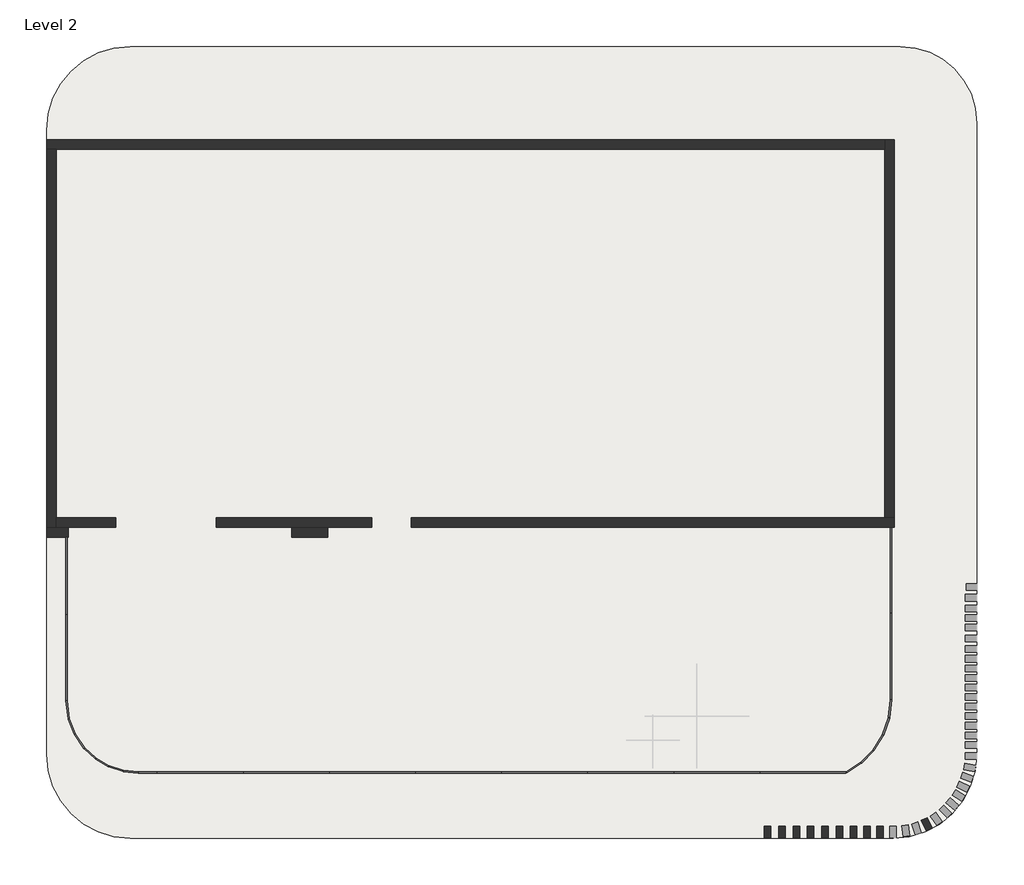
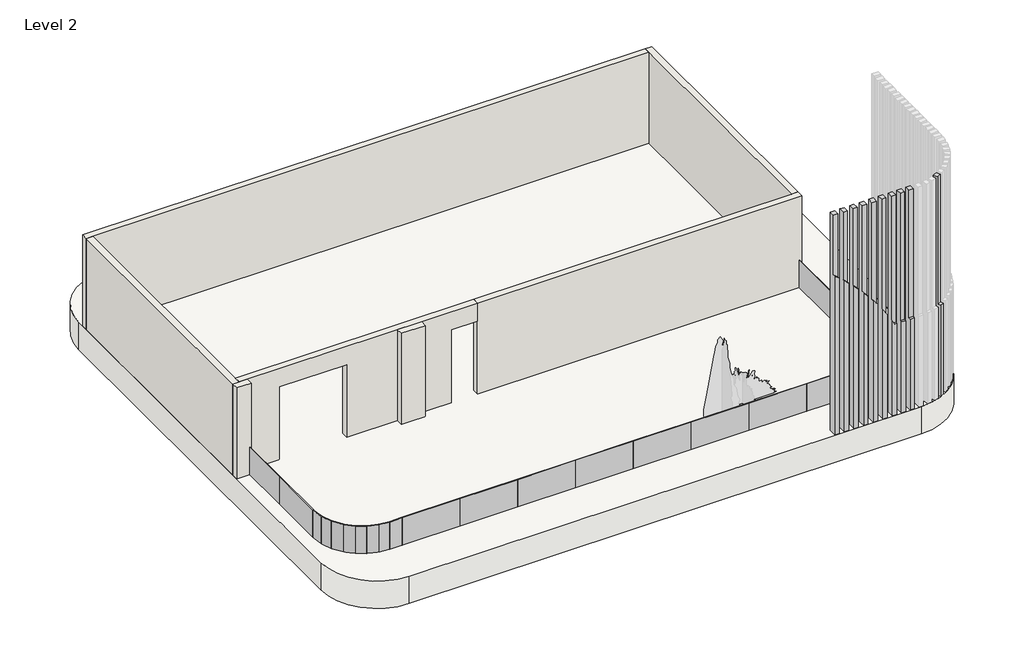
# One storey, part 1 of 2: 25 plates, 10 columns, 7 walls, 1 slab.
"""IFC4 building model written with IfcOpenShell, lengths in millimetres."""

from ifc_helpers import new_model, si_unit, point, frame, frame_2d, origin, place, context, project, spatial, polyline, circle_curve, trimmed, segment, composite_curve, outline, extrude, faceted_brep, transform, mapped, element, save
from ifc_brep_helpers import plane_surface, cylinder_surface, advanced_brep
from components import system_panel_glazed_95be5de7, system_panel_glazed_8746fe8c, system_panel_glazed_ac9e41bb, system_panel_glazed_e5de8428, system_panel_glazed_70ef586e, system_panel_glazed_2e848b93, system_panel_glazed_d6f392a9, system_panel_glazed_76d2efde, system_panel_glazed_f6735284, system_panel_glazed_f2dc5d49, system_panel_glazed_309beea3

model = new_model("IFC4")

# Units and contexts
model_context = context("Model", 3, world=origin())
ifc_project = project(units=[si_unit("LENGTHUNIT", "METRE", prefix="MILLI")], contexts=[model_context])

# Site, building, storey
site = spatial("IfcSite", under=ifc_project)
building = spatial("IfcBuilding", under=site)
storey = spatial("IfcBuildingStorey", under=building, Name="Level 2", Elevation=3048.0)

# Columns
placement = place(None, origin())
element("IfcColumn", 1, ObjectType="Wood Timber Column : 6 x 10", at=placement, inside=storey, context=model_context, shape_type="AdvancedBrep", body=[
    advanced_brep(
    [(3096.1411678, -2145.7759451, 3962.4), (2969.5299699, -2204.8157163, 3962.4), (2867.5521834, -1986.1236473, 3962.4), (2994.1633812, -1927.0838761, 3962.4), (3096.1411678, -2145.7759451, 7010.4), (2969.5299699, -2204.8157163, 7010.4), (2930.0130095, -2120.0713212, 7010.4), (2930.0130095, -2120.0713212, 11277.6), (2867.5521834, -1986.1236473, 11277.6), (2994.1633812, -1927.0838761, 11277.6), (3054.4820737, -2056.4377297, 11277.6), (3054.4820737, -2056.4377297, 7010.4)],
    [
        (0, 1),
        (1, 2),
        (2, 3),
        (3, 0),
        (0, 4),
        (4, 5),
        (5, 1),
        (5, 6),
        (6, 7),
        (7, 8),
        (8, 2),
        (8, 9),
        (9, 3),
        (9, 10),
        (10, 11),
        (11, 4),
        (7, 10, circle_curve(frame((2131.8825083, -405.3567338, 11277.6), z_axis=(0.0, 0.0, 1.0), x_axis=(1.0, 0.0, 0.0)), 1891.3641672)),
        (11, 6, circle_curve(frame((2131.8825083, -405.3567338, 7010.4), z_axis=(0.0, 0.0, -1.0), x_axis=(1.0, 0.0, 0.0)), 1891.3641672)),
    ],
    [
        plane_surface(frame((3096.1411678, -2145.7759451, 3962.4), z_axis=(0.0, 0.0, -1.0000000000000002), x_axis=(0.4226182617406989, -0.9063077870366504, 0.0))),
        plane_surface(frame((2969.5299699, -2204.8157163, 11277.6), z_axis=(0.4226182617406989, -0.9063077870366504, 0.0), x_axis=(0.0, 0.0, -1.0))),
        plane_surface(frame((2867.5521834, -1986.1236473, 11277.6), z_axis=(-0.9063077870366504, -0.4226182617406989, 0.0), x_axis=(0.0, 0.0, -1.0))),
        plane_surface(frame((2994.1633812, -1927.0838761, 11277.6), z_axis=(-0.4226182617406989, 0.9063077870366504, 0.0), x_axis=(0.0, 0.0, -1.0))),
        plane_surface(frame((3096.1411678, -2145.7759451, 11277.6), z_axis=(0.9063077870366504, 0.4226182617406989, 0.0), x_axis=(0.0, 0.0, -1.0))),
        plane_surface(frame((3096.1411678, -2145.7759451, 11277.6), z_axis=(0.0, 0.0, 1.0000000000000002), x_axis=(-0.4226182617406989, 0.9063077870366504, 0.0))),
        plane_surface(frame((4226.4466756, -405.3567338, 7010.4), z_axis=(0.0, 0.0, 1.0), x_axis=(0.0, -1.0, 0.0))),
        cylinder_surface(frame((2131.8825083, -405.3567338, 7010.4), z_axis=(0.0, 0.0, -1.0), x_axis=(1.0, 0.0, 0.0)), 1891.3641672),
    ],
    [
        (0, [[1, 2, 3, 4]]),
        (1, [[-1, 5, 6, 7]]),
        (2, [[-2, -7, 8, 9, 10, 11]]),
        (3, [[-3, -11, 12, 13]]),
        (4, [[-4, -13, 14, 15, 16, -5]]),
        (5, [[-12, -10, 17, -14]]),
        (6, [[18, -8, -6, -16]]),
        (7, [[-18, -15, -17, -9]]),
    ],
),
])
element("IfcColumn", 2, ObjectType="Wood Timber Column : 6 x 10", at=placement, inside=storey, context=model_context, shape_type="SweptSolid", body=[
    extrude(outline(polyline([(-2110.3997962, 3962.4), (-2351.6997962, 3962.4), (-2351.6997962, 7010.4), (-2284.9227607, 7010.4), (-2284.9227607, 11277.6), (-2110.3997962, 11277.6), (-2110.3997962, 3962.4)])), frame((1921.3966756, 0.0, 0.0), z_axis=(1.0, 0.0, 0.0), x_axis=(0.0, 1.0, 0.0)), (0.0, 0.0, 1.0), 139.7),
])
element("IfcColumn", 3, ObjectType="Wood Timber Column : 6 x 10", at=placement, inside=storey, context=model_context, shape_type="SweptSolid", body=[
    extrude(outline(polyline([(-2110.3997962, 3962.4), (-2351.6997962, 3962.4), (-2351.6997962, 7010.4), (-2284.9227607, 7010.4), (-2284.9227607, 11277.6), (-2110.3997962, 11277.6), (-2110.3997962, 3962.4)])), frame((1641.9966756, 0.0, 0.0), z_axis=(1.0, 0.0, 0.0), x_axis=(0.0, 1.0, 0.0)), (0.0, 0.0, 1.0), 139.7),
])
element("IfcColumn", 4, ObjectType="Wood Timber Column : 6 x 10", at=placement, inside=storey, context=model_context, shape_type="AdvancedBrep", body=[
    advanced_brep(
    [(1502.2966756, -2351.6997962, 3962.4), (1362.5966756, -2351.6997962, 3962.4), (1362.5966756, -2110.3997962, 3962.4), (1502.2966756, -2110.3997962, 3962.4), (1502.2966756, -2351.6997962, 7010.4), (1434.0173689, -2351.6997962, 7010.4), (1362.5966756, -2351.6997962, 7137.6306228), (1362.5966756, -2284.9227607, 7137.6306228), (1362.5966756, -2284.9227607, 11277.6), (1362.5966756, -2110.3997962, 11277.6), (1502.2966756, -2110.3997962, 11277.6), (1502.2966756, -2284.9227607, 11277.6), (1502.2966756, -2284.9227607, 7010.4), (1434.0173689, -2284.9227607, 7010.4)],
    [
        (0, 1),
        (1, 2),
        (2, 3),
        (3, 0),
        (0, 4),
        (4, 5),
        (5, 6, circle_curve(frame((-5271.5826311, -2351.6997962, 3329.88412), z_axis=(0.0, -1.0, 0.0), x_axis=(-1.0, 0.0, 0.0)), 7649.26588)),
        (6, 1),
        (6, 7),
        (7, 8),
        (8, 9),
        (9, 2),
        (9, 10),
        (10, 3),
        (10, 11),
        (11, 12),
        (12, 4),
        (8, 11),
        (7, 13, circle_curve(frame((-5271.5826311, -2284.9227607, 3329.88412), z_axis=(0.0, 1.0, 0.0), x_axis=(-1.0, 0.0, 0.0)), 7649.26588)),
        (13, 12),
        (5, 13),
    ],
    [
        plane_surface(frame((1502.2966756, -2351.6997962, 3962.4), z_axis=(0.0, 0.0, -1.0), x_axis=(0.0, -1.0, 0.0))),
        plane_surface(frame((1362.5966756, -2351.6997962, 11277.6), z_axis=(0.0, -1.0, 0.0), x_axis=(0.0, 0.0, -1.0))),
        plane_surface(frame((1362.5966756, -2110.3997962, 11277.6), z_axis=(-1.0, 0.0, 0.0), x_axis=(0.0, 0.0, -1.0))),
        plane_surface(frame((1502.2966756, -2110.3997962, 11277.6), z_axis=(0.0, 1.0, 0.0), x_axis=(0.0, 0.0, -1.0))),
        plane_surface(frame((1502.2966756, -2351.6997962, 11277.6), z_axis=(1.0, 0.0, 0.0), x_axis=(0.0, 0.0, -1.0))),
        plane_surface(frame((1502.2966756, -2351.6997962, 11277.6), z_axis=(0.0, 0.0, 1.0), x_axis=(0.0, 1.0, 0.0))),
        plane_surface(frame((-5271.5826311, -2284.9227607, 10979.15), z_axis=(0.0, -1.0, 0.0), x_axis=(-1.0, 0.0, 0.0))),
        cylinder_surface(frame((-5271.5826311, -2284.9227607, 3329.88412), z_axis=(0.0, 1.0, 0.0), x_axis=(-1.0, 0.0, 0.0)), 7649.26588),
        plane_surface(frame((1434.0173689, -2488.1227607, 7010.4), z_axis=(0.0, 0.0, 1.0), x_axis=(0.0, 1.0, 0.0))),
    ],
    [
        (0, [[1, 2, 3, 4]]),
        (1, [[-1, 5, 6, 7, 8]]),
        (2, [[-2, -8, 9, 10, 11, 12]]),
        (3, [[-3, -12, 13, 14]]),
        (4, [[-4, -14, 15, 16, 17, -5]]),
        (5, [[-13, -11, 18, -15]]),
        (6, [[19, 20, -16, -18, -10]]),
        (7, [[-19, -9, -7, 21]]),
        (8, [[-20, -21, -6, -17]]),
    ],
),
])
element("IfcColumn", 5, ObjectType="Wood Timber Column : 6 x 10", at=placement, inside=storey, context=model_context, shape_type="AdvancedBrep", body=[
    advanced_brep(
    [(1197.4966756, -2351.6997962, 3962.4), (1057.7966756, -2351.6997962, 3962.4), (1057.7966756, -2110.3997962, 3962.4), (1197.4966756, -2110.3997962, 3962.4), (1197.4966756, -2351.6997962, 7411.8299093), (1057.7966756, -2351.6997962, 7625.2567575), (1057.7966756, -2284.9227607, 7625.2567575), (1057.7966756, -2284.9227607, 11277.6), (1057.7966756, -2110.3997962, 11277.6), (1197.4966756, -2110.3997962, 11277.6), (1197.4966756, -2284.9227607, 11277.6), (1197.4966756, -2284.9227607, 7411.8299093)],
    [
        (0, 1),
        (1, 2),
        (2, 3),
        (3, 0),
        (0, 4),
        (4, 5, circle_curve(frame((-5271.5826311, -2351.6997962, 3329.88412), z_axis=(0.0, -1.0, 0.0), x_axis=(-1.0, 0.0, 0.0)), 7649.26588)),
        (5, 1),
        (5, 6),
        (6, 7),
        (7, 8),
        (8, 2),
        (8, 9),
        (9, 3),
        (9, 10),
        (10, 11),
        (11, 4),
        (7, 10),
        (6, 11, circle_curve(frame((-5271.5826311, -2284.9227607, 3329.88412), z_axis=(0.0, 1.0, 0.0), x_axis=(-1.0, 0.0, 0.0)), 7649.26588)),
    ],
    [
        plane_surface(frame((1197.4966756, -2351.6997962, 3962.4), z_axis=(0.0, 0.0, -1.0), x_axis=(0.0, -1.0, 0.0))),
        plane_surface(frame((1057.7966756, -2351.6997962, 11277.6), z_axis=(0.0, -1.0, 0.0), x_axis=(0.0, 0.0, -1.0))),
        plane_surface(frame((1057.7966756, -2110.3997962, 11277.6), z_axis=(-1.0, 0.0, 0.0), x_axis=(0.0, 0.0, -1.0))),
        plane_surface(frame((1197.4966756, -2110.3997962, 11277.6), z_axis=(0.0, 1.0, 0.0), x_axis=(0.0, 0.0, -1.0))),
        plane_surface(frame((1197.4966756, -2351.6997962, 11277.6), z_axis=(1.0, 0.0, 0.0), x_axis=(0.0, 0.0, -1.0))),
        plane_surface(frame((1197.4966756, -2351.6997962, 11277.6), z_axis=(0.0, 0.0, 1.0), x_axis=(0.0, 1.0, 0.0))),
        plane_surface(frame((-5271.5826311, -2284.9227607, 10979.15), z_axis=(0.0, -1.0, 0.0), x_axis=(-1.0, 0.0, 0.0))),
        cylinder_surface(frame((-5271.5826311, -2284.9227607, 3329.88412), z_axis=(0.0, 1.0, 0.0), x_axis=(-1.0, 0.0, 0.0)), 7649.26588),
    ],
    [
        (0, [[1, 2, 3, 4]]),
        (1, [[-1, 5, 6, 7]]),
        (2, [[-2, -7, 8, 9, 10, 11]]),
        (3, [[-3, -11, 12, 13]]),
        (4, [[-4, -13, 14, 15, 16, -5]]),
        (5, [[-12, -10, 17, -14]]),
        (6, [[18, -15, -17, -9]]),
        (7, [[-18, -8, -6, -16]]),
    ],
),
])
element("IfcColumn", 6, ObjectType="Wood Timber Column : 6 x 10", at=placement, inside=storey, context=model_context, shape_type="AdvancedBrep", body=[
    advanced_brep(
    [(892.6966756, -2351.6997962, 3962.4), (752.9966756, -2351.6997962, 3962.4), (752.9966756, -2110.3997962, 3962.4), (892.6966756, -2110.3997962, 3962.4), (892.6966756, -2351.6997962, 7859.0042478), (752.9966756, -2351.6997962, 8043.2388362), (752.9966756, -2284.9227607, 8043.2388362), (752.9966756, -2284.9227607, 11277.6), (752.9966756, -2110.3997962, 11277.6), (892.6966756, -2110.3997962, 11277.6), (892.6966756, -2284.9227607, 11277.6), (892.6966756, -2284.9227607, 7859.0042478)],
    [
        (0, 1),
        (1, 2),
        (2, 3),
        (3, 0),
        (0, 4),
        (4, 5, circle_curve(frame((-5271.5826311, -2351.6997962, 3329.88412), z_axis=(0.0, -1.0, 0.0), x_axis=(-1.0, 0.0, 0.0)), 7649.26588)),
        (5, 1),
        (5, 6),
        (6, 7),
        (7, 8),
        (8, 2),
        (8, 9),
        (9, 3),
        (9, 10),
        (10, 11),
        (11, 4),
        (7, 10),
        (6, 11, circle_curve(frame((-5271.5826311, -2284.9227607, 3329.88412), z_axis=(0.0, 1.0, 0.0), x_axis=(-1.0, 0.0, 0.0)), 7649.26588)),
    ],
    [
        plane_surface(frame((892.6966756, -2351.6997962, 3962.4), z_axis=(0.0, 0.0, -1.0), x_axis=(0.0, -1.0, 0.0))),
        plane_surface(frame((752.9966756, -2351.6997962, 11277.6), z_axis=(0.0, -1.0, 0.0), x_axis=(0.0, 0.0, -1.0))),
        plane_surface(frame((752.9966756, -2110.3997962, 11277.6), z_axis=(-1.0, 0.0, 0.0), x_axis=(0.0, 0.0, -1.0))),
        plane_surface(frame((892.6966756, -2110.3997962, 11277.6), z_axis=(0.0, 1.0, 0.0), x_axis=(0.0, 0.0, -1.0))),
        plane_surface(frame((892.6966756, -2351.6997962, 11277.6), z_axis=(1.0, 0.0, 0.0), x_axis=(0.0, 0.0, -1.0))),
        plane_surface(frame((892.6966756, -2351.6997962, 11277.6), z_axis=(0.0, 0.0, 1.0), x_axis=(0.0, 1.0, 0.0))),
        plane_surface(frame((-5271.5826311, -2284.9227607, 10979.15), z_axis=(0.0, -1.0, 0.0), x_axis=(-1.0, 0.0, 0.0))),
        cylinder_surface(frame((-5271.5826311, -2284.9227607, 3329.88412), z_axis=(0.0, 1.0, 0.0), x_axis=(-1.0, 0.0, 0.0)), 7649.26588),
    ],
    [
        (0, [[1, 2, 3, 4]]),
        (1, [[-1, 5, 6, 7]]),
        (2, [[-2, -7, 8, 9, 10, 11]]),
        (3, [[-3, -11, 12, 13]]),
        (4, [[-4, -13, 14, 15, 16, -5]]),
        (5, [[-12, -10, 17, -14]]),
        (6, [[18, -15, -17, -9]]),
        (7, [[-18, -8, -6, -16]]),
    ],
),
])
element("IfcColumn", 7, ObjectType="Wood Timber Column : 6 x 10", at=placement, inside=storey, context=model_context, shape_type="AdvancedBrep", body=[
    advanced_brep(
    [(587.8966756, -2351.6997962, 3962.4), (448.1966756, -2351.6997962, 3962.4), (448.1966756, -2110.3997962, 3962.4), (587.8966756, -2110.3997962, 3962.4), (587.8966756, -2351.6997962, 8246.9737834), (448.1966756, -2351.6997962, 8408.8006566), (448.1966756, -2284.9227607, 8408.8006566), (448.1966756, -2284.9227607, 11277.6), (448.1966756, -2110.3997962, 11277.6), (587.8966756, -2110.3997962, 11277.6), (587.8966756, -2284.9227607, 11277.6), (587.8966756, -2284.9227607, 8246.9737834)],
    [
        (0, 1),
        (1, 2),
        (2, 3),
        (3, 0),
        (0, 4),
        (4, 5, circle_curve(frame((-5271.5826311, -2351.6997962, 3329.88412), z_axis=(0.0, -1.0, 0.0), x_axis=(-1.0, 0.0, 0.0)), 7649.26588)),
        (5, 1),
        (5, 6),
        (6, 7),
        (7, 8),
        (8, 2),
        (8, 9),
        (9, 3),
        (9, 10),
        (10, 11),
        (11, 4),
        (7, 10),
        (6, 11, circle_curve(frame((-5271.5826311, -2284.9227607, 3329.88412), z_axis=(0.0, 1.0, 0.0), x_axis=(-1.0, 0.0, 0.0)), 7649.26588)),
    ],
    [
        plane_surface(frame((587.8966756, -2351.6997962, 3962.4), z_axis=(0.0, 0.0, -1.0), x_axis=(0.0, -1.0, 0.0))),
        plane_surface(frame((448.1966756, -2351.6997962, 11277.6), z_axis=(0.0, -1.0, 0.0), x_axis=(0.0, 0.0, -1.0))),
        plane_surface(frame((448.1966756, -2110.3997962, 11277.6), z_axis=(-1.0, 0.0, 0.0), x_axis=(0.0, 0.0, -1.0))),
        plane_surface(frame((587.8966756, -2110.3997962, 11277.6), z_axis=(0.0, 1.0, 0.0), x_axis=(0.0, 0.0, -1.0))),
        plane_surface(frame((587.8966756, -2351.6997962, 11277.6), z_axis=(1.0, 0.0, 0.0), x_axis=(0.0, 0.0, -1.0))),
        plane_surface(frame((587.8966756, -2351.6997962, 11277.6), z_axis=(0.0, 0.0, 1.0), x_axis=(0.0, 1.0, 0.0))),
        plane_surface(frame((-5271.5826311, -2284.9227607, 10979.15), z_axis=(0.0, -1.0, 0.0), x_axis=(-1.0, 0.0, 0.0))),
        cylinder_surface(frame((-5271.5826311, -2284.9227607, 3329.88412), z_axis=(0.0, 1.0, 0.0), x_axis=(-1.0, 0.0, 0.0)), 7649.26588),
    ],
    [
        (0, [[1, 2, 3, 4]]),
        (1, [[-1, 5, 6, 7]]),
        (2, [[-2, -7, 8, 9, 10, 11]]),
        (3, [[-3, -11, 12, 13]]),
        (4, [[-4, -13, 14, 15, 16, -5]]),
        (5, [[-12, -10, 17, -14]]),
        (6, [[18, -15, -17, -9]]),
        (7, [[-18, -8, -6, -16]]),
    ],
),
])
element("IfcColumn", 8, ObjectType="Wood Timber Column : 6 x 10", at=placement, inside=storey, context=model_context, shape_type="AdvancedBrep", body=[
    advanced_brep(
    [(283.0966756, -2351.6997962, 3962.4), (143.3966756, -2351.6997962, 3962.4), (143.3966756, -2110.3997962, 3962.4), (283.0966756, -2110.3997962, 3962.4), (283.0966756, -2351.6997962, 8588.8580031), (143.3966756, -2351.6997962, 8732.5934043), (143.3966756, -2284.9227607, 8732.5934043), (143.3966756, -2284.9227607, 11277.6), (143.3966756, -2110.3997962, 11277.6), (283.0966756, -2110.3997962, 11277.6), (283.0966756, -2284.9227607, 11277.6), (283.0966756, -2284.9227607, 8588.8580031)],
    [
        (0, 1),
        (1, 2),
        (2, 3),
        (3, 0),
        (0, 4),
        (4, 5, circle_curve(frame((-5271.5826311, -2351.6997962, 3329.88412), z_axis=(0.0, -1.0, 0.0), x_axis=(-1.0, 0.0, 0.0)), 7649.26588)),
        (5, 1),
        (5, 6),
        (6, 7),
        (7, 8),
        (8, 2),
        (8, 9),
        (9, 3),
        (9, 10),
        (10, 11),
        (11, 4),
        (7, 10),
        (6, 11, circle_curve(frame((-5271.5826311, -2284.9227607, 3329.88412), z_axis=(0.0, 1.0, 0.0), x_axis=(-1.0, 0.0, 0.0)), 7649.26588)),
    ],
    [
        plane_surface(frame((283.0966756, -2351.6997962, 3962.4), z_axis=(0.0, 0.0, -1.0), x_axis=(0.0, -1.0, 0.0))),
        plane_surface(frame((143.3966756, -2351.6997962, 11277.6), z_axis=(0.0, -1.0, 0.0), x_axis=(0.0, 0.0, -1.0))),
        plane_surface(frame((143.3966756, -2110.3997962, 11277.6), z_axis=(-1.0, 0.0, 0.0), x_axis=(0.0, 0.0, -1.0))),
        plane_surface(frame((283.0966756, -2110.3997962, 11277.6), z_axis=(0.0, 1.0, 0.0), x_axis=(0.0, 0.0, -1.0))),
        plane_surface(frame((283.0966756, -2351.6997962, 11277.6), z_axis=(1.0, 0.0, 0.0), x_axis=(0.0, 0.0, -1.0))),
        plane_surface(frame((283.0966756, -2351.6997962, 11277.6), z_axis=(0.0, 0.0, 1.0), x_axis=(0.0, 1.0, 0.0))),
        plane_surface(frame((-5271.5826311, -2284.9227607, 10979.15), z_axis=(0.0, -1.0, 0.0), x_axis=(-1.0, 0.0, 0.0))),
        cylinder_surface(frame((-5271.5826311, -2284.9227607, 3329.88412), z_axis=(0.0, 1.0, 0.0), x_axis=(-1.0, 0.0, 0.0)), 7649.26588),
    ],
    [
        (0, [[1, 2, 3, 4]]),
        (1, [[-1, 5, 6, 7]]),
        (2, [[-2, -7, 8, 9, 10, 11]]),
        (3, [[-3, -11, 12, 13]]),
        (4, [[-4, -13, 14, 15, 16, -5]]),
        (5, [[-12, -10, 17, -14]]),
        (6, [[18, -15, -17, -9]]),
        (7, [[-18, -8, -6, -16]]),
    ],
),
])
element("IfcColumn", 9, ObjectType="Wood Timber Column : 6 x 10", at=placement, inside=storey, context=model_context, shape_type="AdvancedBrep", body=[
    advanced_brep(
    [(-21.7033244, -2351.6997962, 3962.4), (-161.4033244, -2351.6997962, 3962.4), (-161.4033244, -2110.3997962, 3962.4), (-21.7033244, -2110.3997962, 3962.4), (-21.7033244, -2351.6997962, 8893.1597529), (-161.4033244, -2351.6997962, 9021.7498911), (-161.4033244, -2284.9227607, 9021.7498911), (-161.4033244, -2284.9227607, 11277.6), (-161.4033244, -2110.3997962, 11277.6), (-21.7033244, -2110.3997962, 11277.6), (-21.7033244, -2284.9227607, 11277.6), (-21.7033244, -2284.9227607, 8893.1597529)],
    [
        (0, 1),
        (1, 2),
        (2, 3),
        (3, 0),
        (0, 4),
        (4, 5, circle_curve(frame((-5271.5826311, -2351.6997962, 3329.88412), z_axis=(0.0, -1.0, 0.0), x_axis=(-1.0, 0.0, 0.0)), 7649.26588)),
        (5, 1),
        (5, 6),
        (6, 7),
        (7, 8),
        (8, 2),
        (8, 9),
        (9, 3),
        (9, 10),
        (10, 11),
        (11, 4),
        (7, 10),
        (6, 11, circle_curve(frame((-5271.5826311, -2284.9227607, 3329.88412), z_axis=(0.0, 1.0, 0.0), x_axis=(-1.0, 0.0, 0.0)), 7649.26588)),
    ],
    [
        plane_surface(frame((-21.7033244, -2351.6997962, 3962.4), z_axis=(0.0, 0.0, -1.0), x_axis=(0.0, -1.0, 0.0))),
        plane_surface(frame((-161.4033244, -2351.6997962, 11277.6), z_axis=(0.0, -1.0, 0.0), x_axis=(0.0, 0.0, -1.0))),
        plane_surface(frame((-161.4033244, -2110.3997962, 11277.6), z_axis=(-1.0, 0.0, 0.0), x_axis=(0.0, 0.0, -1.0))),
        plane_surface(frame((-21.7033244, -2110.3997962, 11277.6), z_axis=(0.0, 1.0, 0.0), x_axis=(0.0, 0.0, -1.0))),
        plane_surface(frame((-21.7033244, -2351.6997962, 11277.6), z_axis=(1.0, 0.0, 0.0), x_axis=(0.0, 0.0, -1.0))),
        plane_surface(frame((-21.7033244, -2351.6997962, 11277.6), z_axis=(0.0, 0.0, 1.0), x_axis=(0.0, 1.0, 0.0))),
        plane_surface(frame((-5271.5826311, -2284.9227607, 10979.15), z_axis=(0.0, -1.0, 0.0), x_axis=(-1.0, 0.0, 0.0))),
        cylinder_surface(frame((-5271.5826311, -2284.9227607, 3329.88412), z_axis=(0.0, 1.0, 0.0), x_axis=(-1.0, 0.0, 0.0)), 7649.26588),
    ],
    [
        (0, [[1, 2, 3, 4]]),
        (1, [[-1, 5, 6, 7]]),
        (2, [[-2, -7, 8, 9, 10, 11]]),
        (3, [[-3, -11, 12, 13]]),
        (4, [[-4, -13, 14, 15, 16, -5]]),
        (5, [[-12, -10, 17, -14]]),
        (6, [[18, -15, -17, -9]]),
        (7, [[-18, -8, -6, -16]]),
    ],
),
])
element("IfcColumn", 10, ObjectType="Wood Timber Column : 6 x 10", at=placement, inside=storey, context=model_context, shape_type="AdvancedBrep", body=[
    advanced_brep(
    [(-326.5033244, -2351.6997962, 3962.4), (-466.2033244, -2351.6997962, 3962.4), (-466.2033244, -2110.3997962, 3962.4), (-326.5033244, -2110.3997962, 3962.4), (-326.5033244, -2351.6997962, 9165.7610167), (-466.2033244, -2351.6997962, 9281.3207719), (-466.2033244, -2284.9227607, 9281.3207719), (-466.2033244, -2284.9227607, 11277.6), (-466.2033244, -2110.3997962, 11277.6), (-326.5033244, -2110.3997962, 11277.6), (-326.5033244, -2284.9227607, 11277.6), (-326.5033244, -2284.9227607, 9165.7610167)],
    [
        (0, 1),
        (1, 2),
        (2, 3),
        (3, 0),
        (0, 4),
        (4, 5, circle_curve(frame((-5271.5826311, -2351.6997962, 3329.88412), z_axis=(0.0, -1.0, 0.0), x_axis=(-1.0, 0.0, 0.0)), 7649.26588)),
        (5, 1),
        (5, 6),
        (6, 7),
        (7, 8),
        (8, 2),
        (8, 9),
        (9, 3),
        (9, 10),
        (10, 11),
        (11, 4),
        (7, 10),
        (6, 11, circle_curve(frame((-5271.5826311, -2284.9227607, 3329.88412), z_axis=(0.0, 1.0, 0.0), x_axis=(-1.0, 0.0, 0.0)), 7649.26588)),
    ],
    [
        plane_surface(frame((-326.5033244, -2351.6997962, 3962.4), z_axis=(0.0, 0.0, -1.0), x_axis=(0.0, -1.0, 0.0))),
        plane_surface(frame((-466.2033244, -2351.6997962, 11277.6), z_axis=(0.0, -1.0, 0.0), x_axis=(0.0, 0.0, -1.0))),
        plane_surface(frame((-466.2033244, -2110.3997962, 11277.6), z_axis=(-1.0, 0.0, 0.0), x_axis=(0.0, 0.0, -1.0))),
        plane_surface(frame((-326.5033244, -2110.3997962, 11277.6), z_axis=(0.0, 1.0, 0.0), x_axis=(0.0, 0.0, -1.0))),
        plane_surface(frame((-326.5033244, -2351.6997962, 11277.6), z_axis=(1.0, 0.0, 0.0), x_axis=(0.0, 0.0, -1.0))),
        plane_surface(frame((-326.5033244, -2351.6997962, 11277.6), z_axis=(0.0, 0.0, 1.0), x_axis=(0.0, 1.0, 0.0))),
        plane_surface(frame((-5271.5826311, -2284.9227607, 10979.15), z_axis=(0.0, -1.0, 0.0), x_axis=(-1.0, 0.0, 0.0))),
        cylinder_surface(frame((-5271.5826311, -2284.9227607, 3329.88412), z_axis=(0.0, 1.0, 0.0), x_axis=(-1.0, 0.0, 0.0)), 7649.26588),
    ],
    [
        (0, [[1, 2, 3, 4]]),
        (1, [[-1, 5, 6, 7]]),
        (2, [[-2, -7, 8, 9, 10, 11]]),
        (3, [[-3, -11, 12, 13]]),
        (4, [[-4, -13, 14, 15, 16, -5]]),
        (5, [[-12, -10, 17, -14]]),
        (6, [[18, -15, -17, -9]]),
        (7, [[-18, -8, -6, -16]]),
    ],
),
])

# Plates
system_panel_glazed_shape = system_panel_glazed_95be5de7(model_context)
element("IfcPlate", 11, ObjectType="System Panel : Glazed", at=placement, inside=storey, context=model_context, shape_type="MappedRepresentation", body=[
    mapped(system_panel_glazed_shape, transform((2194.4466756, 3328.5792748, 3962.4), x_axis=(0.0, -1.0, 0.0), y_axis=(1.0, 0.0, 0.0), z_axis=(0.0, 0.0, 1.0))),
])
element("IfcPlate", 12, ObjectType="System Panel : Glazed", at=placement, inside=storey, context=model_context, shape_type="MappedRepresentation", body=[
    mapped(system_panel_glazed_shape, transform((2194.4466756, 1499.7792748, 3962.4), x_axis=(0.0, -1.0, 0.0), y_axis=(1.0, 0.0, 0.0), z_axis=(0.0, 0.0, 1.0))),
])
element("IfcPlate", 13, ObjectType="System Panel : Glazed", at=placement, inside=storey, context=model_context, shape_type="MappedRepresentation", body=[
    mapped(system_panel_glazed_shape, transform((349.2738683, -935.6497962, 3962.4), x_axis=(-1.0, 0.0, 0.0), y_axis=(0.0, -1.0, 0.0), z_axis=(0.0, 0.0, 1.0))),
])
element("IfcPlate", 14, ObjectType="System Panel : Glazed", at=placement, inside=storey, context=model_context, shape_type="MappedRepresentation", body=[
    mapped(system_panel_glazed_shape, transform((-1479.5261317, -935.6497962, 3962.4), x_axis=(-1.0, 0.0, 0.0), y_axis=(0.0, -1.0, 0.0), z_axis=(0.0, 0.0, 1.0))),
])
element("IfcPlate", 15, ObjectType="System Panel : Glazed", at=placement, inside=storey, context=model_context, shape_type="MappedRepresentation", body=[
    mapped(system_panel_glazed_shape, transform((-3308.3261317, -935.6497962, 3962.4), x_axis=(-1.0, 0.0, 0.0), y_axis=(0.0, -1.0, 0.0), z_axis=(0.0, 0.0, 1.0))),
])
element("IfcPlate", 16, ObjectType="System Panel : Glazed", at=placement, inside=storey, context=model_context, shape_type="MappedRepresentation", body=[
    mapped(system_panel_glazed_shape, transform((-5137.1261317, -935.6497962, 3962.4), x_axis=(-1.0, 0.0, 0.0), y_axis=(0.0, -1.0, 0.0), z_axis=(0.0, 0.0, 1.0))),
])
element("IfcPlate", 17, ObjectType="System Panel : Glazed", at=placement, inside=storey, context=model_context, shape_type="MappedRepresentation", body=[
    mapped(system_panel_glazed_shape, transform((-6965.9261317, -935.6497962, 3962.4), x_axis=(-1.0, 0.0, 0.0), y_axis=(0.0, -1.0, 0.0), z_axis=(0.0, 0.0, 1.0))),
])
element("IfcPlate", 18, ObjectType="System Panel : Glazed", at=placement, inside=storey, context=model_context, shape_type="MappedRepresentation", body=[
    mapped(system_panel_glazed_shape, transform((-8794.7261317, -935.6497962, 3962.4), x_axis=(-1.0, 0.0, 0.0), y_axis=(0.0, -1.0, 0.0), z_axis=(0.0, 0.0, 1.0))),
])
element("IfcPlate", 19, ObjectType="System Panel : Glazed", at=placement, inside=storey, context=model_context, shape_type="MappedRepresentation", body=[
    mapped(system_panel_glazed_shape, transform((-10623.5261317, -935.6497962, 3962.4), x_axis=(-1.0, 0.0, 0.0), y_axis=(0.0, -1.0, 0.0), z_axis=(0.0, 0.0, 1.0))),
])
element("IfcPlate", 20, ObjectType="System Panel : Glazed", at=placement, inside=storey, context=model_context, shape_type="MappedRepresentation", body=[
    mapped(system_panel_glazed_shape, transform((-15257.878953, 1474.2432662, 3962.4), x_axis=(0.0, 1.0, 0.0), y_axis=(-1.0, 0.0, 0.0), z_axis=(0.0, 0.0, 1.0))),
])
element("IfcPlate", 21, ObjectType="System Panel : Glazed", at=placement, inside=storey, context=model_context, shape_type="MappedRepresentation", body=[
    mapped(system_panel_glazed_shape, transform((-12452.3261317, -935.6497962, 3962.4), x_axis=(-1.0, 0.0, 0.0), y_axis=(0.0, -1.0, 0.0), z_axis=(0.0, 0.0, 1.0))),
])
system_panel_glazed_2_shape = system_panel_glazed_8746fe8c(model_context)
element("IfcPlate", 22, ObjectType="System Panel : Glazed", at=placement, inside=storey, context=model_context, shape_type="MappedRepresentation", body=[
    mapped(system_panel_glazed_2_shape, transform((-15233.6907484, 371.1948552, 3962.4), x_axis=(-0.12717730440498604, 0.9918799994174101, 0.0), y_axis=(-0.9918799994174101, -0.12717730440498604, 0.0), z_axis=(0.0, 0.0, 1.0))),
])
system_panel_glazed_3_shape = system_panel_glazed_ac9e41bb(model_context)
element("IfcPlate", 23, ObjectType="System Panel : Glazed", at=placement, inside=storey, context=model_context, shape_type="MappedRepresentation", body=[
    mapped(system_panel_glazed_3_shape, transform((1693.1791797, -610.1817883, 3962.4), x_axis=(-0.7037559478689831, -0.7104418103117449, 0.0), y_axis=(0.7104418103117449, -0.7037559478689831, 0.0), z_axis=(0.0, 0.0, 1.0))),
])
system_panel_glazed_4_shape = system_panel_glazed_e5de8428(model_context)
element("IfcPlate", 24, ObjectType="System Panel : Glazed", at=placement, inside=storey, context=model_context, shape_type="MappedRepresentation", body=[
    mapped(system_panel_glazed_4_shape, transform((2172.8580572, 394.5617647, 3962.4), x_axis=(-0.11242030431559506, -0.9936607445087026, 0.0), y_axis=(0.9936607445087026, -0.11242030431559506, 0.0), z_axis=(0.0, 0.0, 1.0))),
])
element("IfcPlate", 25, ObjectType="System Panel : Glazed", at=placement, inside=storey, context=model_context, shape_type="MappedRepresentation", body=[
    mapped(system_panel_glazed_4_shape, transform((1921.3790958, -320.9636625, 3962.4), x_axis=(-0.533972740511033, -0.8455016927192618, 0.0), y_axis=(0.8455016927192618, -0.533972740511033, 0.0), z_axis=(0.0, 0.0, 1.0))),
])
element("IfcPlate", 26, ObjectType="System Panel : Glazed", at=placement, inside=storey, context=model_context, shape_type="MappedRepresentation", body=[
    mapped(system_panel_glazed_4_shape, transform((2087.5949598, 22.5731991, 3962.4), x_axis=(-0.3315776956564623, -0.943427915499192, 0.0), y_axis=(0.943427915499192, -0.3315776956564623, 0.0), z_axis=(0.0, 0.0, 1.0))),
])
system_panel_glazed_5_shape = system_panel_glazed_70ef586e(model_context)
element("IfcPlate", 27, ObjectType="System Panel : Glazed", at=placement, inside=storey, context=model_context, shape_type="MappedRepresentation", body=[
    mapped(system_panel_glazed_5_shape, transform((-15148.5211317, 24.6162823, 3962.4), x_axis=(-0.3602087986279214, 0.9328717068230924, 0.0), y_axis=(-0.9328717068230924, -0.3602087986279214, 0.0), z_axis=(0.0, 0.0, 1.0))),
])
system_panel_glazed_6_shape = system_panel_glazed_2e848b93(model_context)
element("IfcPlate", 28, ObjectType="System Panel : Glazed", at=placement, inside=storey, context=model_context, shape_type="MappedRepresentation", body=[
    mapped(system_panel_glazed_6_shape, transform((-14984.0134084, -283.3108779, 3962.4), x_axis=(-0.5680307758785693, 0.8230073132450225, 0.0), y_axis=(-0.8230073132450225, -0.5680307758785693, 0.0), z_axis=(0.0, 0.0, 1.0))),
])
system_panel_glazed_7_shape = system_panel_glazed_d6f392a9(model_context)
element("IfcPlate", 29, ObjectType="System Panel : Glazed", at=placement, inside=storey, context=model_context, shape_type="MappedRepresentation", body=[
    mapped(system_panel_glazed_7_shape, transform((-14765.0266334, -538.6896648, 3962.4), x_axis=(-0.7386085467399861, 0.6741345671916296, 0.0), y_axis=(-0.6741345671916296, -0.7386085467399861, 0.0), z_axis=(0.0, 0.0, 1.0))),
])
system_panel_glazed_8_shape = system_panel_glazed_76d2efde(model_context)
element("IfcPlate", 30, ObjectType="System Panel : Glazed", at=placement, inside=storey, context=model_context, shape_type="MappedRepresentation", body=[
    mapped(system_panel_glazed_8_shape, transform((-13919.4974005, -918.9578788, 3962.4), x_axis=(-0.994403599652405, 0.10564791052519472, 0.0), y_axis=(-0.10564791052519472, -0.994403599652405, 0.0), z_axis=(0.0, 0.0, 1.0))),
])
element("IfcPlate", 31, ObjectType="System Panel : Glazed", at=placement, inside=storey, context=model_context, shape_type="MappedRepresentation", body=[
    mapped(system_panel_glazed_8_shape, transform((-14513.1846616, -723.8381812, 3962.4), x_axis=(-0.8631975005225224, 0.5048663933078434, 0.0), y_axis=(-0.5048663933078434, -0.8631975005225224, 0.0), z_axis=(0.0, 0.0, 1.0))),
])
element("IfcPlate", 32, ObjectType="System Panel : Glazed", at=placement, inside=storey, context=model_context, shape_type="MappedRepresentation", body=[
    mapped(system_panel_glazed_8_shape, transform((-14226.7060319, -852.9354353, 3962.4), x_axis=(-0.950007532123609, 0.31222698299219753, 0.0), y_axis=(-0.31222698299219753, -0.950007532123609, 0.0), z_axis=(0.0, 0.0, 1.0))),
])
system_panel_glazed_9_shape = system_panel_glazed_f6735284(model_context)
element("IfcPlate", 33, ObjectType="System Panel : Glazed", at=placement, inside=storey, context=model_context, shape_type="MappedRepresentation", body=[
    mapped(system_panel_glazed_9_shape, transform((-15257.878953, 3207.8612705, 3962.4), x_axis=(0.0, 1.0, 0.0), y_axis=(-1.0, 0.0, 0.0), z_axis=(0.0, 0.0, 1.0))),
])
system_panel_glazed_10_shape = system_panel_glazed_f2dc5d49(model_context)
element("IfcPlate", 34, ObjectType="System Panel : Glazed", at=placement, inside=storey, context=model_context, shape_type="MappedRepresentation", body=[
    mapped(system_panel_glazed_10_shape, transform((1415.5972584, -836.3419521, 3962.4), x_axis=(-0.8370369368070523, -0.5471463848191513, 0.0), y_axis=(0.5471463848191513, -0.8370369368070523, 0.0), z_axis=(0.0, 0.0, 1.0))),
])
system_panel_glazed_11_shape = system_panel_glazed_309beea3(model_context)
element("IfcPlate", 35, ObjectType="System Panel : Glazed", at=placement, inside=storey, context=model_context, shape_type="MappedRepresentation", body=[
    mapped(system_panel_glazed_11_shape, transform((-13564.5560112, -935.6497962, 3962.4), x_axis=(-1.0, 0.0, 0.0), y_axis=(0.0, -1.0, 0.0), z_axis=(0.0, 0.0, 1.0))),
])

# Slab
element("IfcSlab", 36, ObjectType="Generic - 3'", at=placement, inside=storey, context=model_context, shape_type="SweptSolid", body=[
    extrude(outline(composite_curve([segment(trimmed(circle_curve(frame_2d((2423.0466756, 12828.0432662)), 1625.6), [point((2423.0466756, 14453.6432662))], [point((4048.6466756, 12828.0432662))], False, "CARTESIAN"), True, "CONTINUOUS"), segment(polyline([(4048.6466756, 12828.0432662), (4048.6466756, -583.1567338)]), True, "CONTINUOUS"), segment(trimmed(circle_curve(frame_2d((2270.6466756, -583.1567338)), 1778.0), [point((4048.6466756, -583.1567338))], [point((2270.6466756, -2361.1567338))], False, "CARTESIAN"), True, "CONTINUOUS"), segment(polyline([(2270.6466756, -2361.1567338), (-13934.5533244, -2361.1567338)]), True, "CONTINUOUS"), segment(trimmed(circle_curve(frame_2d((-13934.5533244, -583.1567338)), 1778.0), [point((-13934.5533244, -2361.1567338))], [point((-15712.5533244, -583.1567338))], False, "CARTESIAN"), True, "CONTINUOUS"), segment(polyline([(-15712.5533244, -583.1567338), (-15712.5533244, 12675.6432662)]), True, "CONTINUOUS"), segment(trimmed(circle_curve(frame_2d((-13934.5533244, 12675.6432662)), 1778.0), [point((-15712.5533244, 12675.6432662))], [point((-13934.5533244, 14453.6432662))], False, "CARTESIAN"), True, "CONTINUOUS"), segment(polyline([(-13934.5533244, 14453.6432662), (2423.0466756, 14453.6432662)]), True, "CONTINUOUS")], self_intersect=False)), frame((0.0, 0.0, 3048.0), z_axis=(0.0, 0.0, 1.0), x_axis=(1.0, 0.0, 0.0)), (0.0, 0.0, 1.0), 914.4),
])

# Walls
element("IfcWall", 37, ObjectType="Generic - 8\" brown", at=placement, inside=storey, context=model_context, shape_type="SweptSolid", body=[
    extrude(outline(polyline([(-15255.3533244, 4027.0792748), (-15712.5533244, 4027.0792748), (-15712.5533244, 4230.2792748), (-15255.3533244, 4230.2792748), (-15255.3533244, 4027.0792748)])), frame((0.0, 0.0, 3962.4), z_axis=(0.0, 0.0, 1.0), x_axis=(1.0, 0.0, 0.0)), (0.0, 0.0, 1.0), 3048.0),
])
element("IfcWall", 38, ObjectType="Generic - 8\" brown", at=placement, inside=storey, context=model_context, shape_type="SweptSolid", body=[
    extrude(outline(polyline([(-9743.5533244, 4027.0792748), (-10505.5533244, 4027.0792748), (-10505.5533244, 4230.2792748), (-9743.5533244, 4230.2792748), (-9743.5533244, 4027.0792748)])), frame((0.0, 0.0, 3962.4), z_axis=(0.0, 0.0, 1.0), x_axis=(1.0, 0.0, 0.0)), (0.0, 0.0, 1.0), 3048.0),
])
element("IfcWall", 39, ObjectType="Generic - 8\" wood", at=placement, inside=storey, context=model_context, shape_type="Brep", body=[
    faceted_brep([(-15712.5533244, 12269.3792748, 3962.4), (-15509.3533244, 12269.3792748, 3962.4), (2092.8466756, 12269.3792748, 3962.4), (2092.8466756, 12269.3792748, 7010.4), (-15509.3533244, 12269.3792748, 7010.4), (-15712.5533244, 12269.3792748, 7010.4), (-15712.5533244, 12472.5792748, 3962.4), (-15712.5533244, 12472.5792748, 7010.4), (2092.8466756, 12472.5792748, 7010.4), (2092.8466756, 12472.5792748, 3962.4)], [[[0, 1, 2, 3, 4, 5]], [[6, 7, 8, 9]], [[2, 1, 0, 6, 9]], [[5, 4, 3, 8, 7]], [[0, 5, 7, 6]], [[3, 2, 9, 8]]]),
])
element("IfcWall", 40, ObjectType="Generic - 8\" wood", at=placement, inside=storey, context=model_context, shape_type="Brep", body=[
    faceted_brep([(-15509.3533244, 4242.9792748, 3962.4), (-15509.3533244, 4446.1792748, 3962.4), (-15509.3533244, 12269.3792748, 3962.4), (-15509.3533244, 12269.3792748, 7010.4), (-15509.3533244, 4446.1792748, 7010.4), (-15509.3533244, 4242.9792748, 7010.4), (-15712.5533244, 4242.9792748, 3962.4), (-15712.5533244, 4242.9792748, 7010.4), (-15712.5533244, 12269.3792748, 7010.4), (-15712.5533244, 12269.3792748, 3962.4)], [[[0, 1, 2, 3, 4, 5]], [[6, 7, 8, 9]], [[2, 1, 0, 6, 9]], [[5, 4, 3, 8, 7]], [[0, 5, 7, 6]], [[3, 2, 9, 8]]]),
])
element("IfcWall", 41, ObjectType="Generic - 8\" wood", at=placement, inside=storey, context=model_context, shape_type="Brep", body=[
    faceted_brep([(2092.8466756, 12472.5792748, 3962.4), (2092.8466756, 12269.3792748, 3962.4), (2092.8466756, 4446.1792748, 3962.4), (2092.8466756, 4446.1792748, 7010.4), (2092.8466756, 12269.3792748, 7010.4), (2092.8466756, 12472.5792748, 7010.4), (2296.0466756, 12472.5792748, 3962.4), (2296.0466756, 12472.5792748, 7010.4), (2296.0466756, 4446.1792748, 7010.4), (2296.0466756, 4446.1792748, 3962.4)], [[[0, 1, 2, 3, 4, 5]], [[6, 7, 8, 9]], [[2, 1, 0, 6, 9]], [[5, 4, 3, 8, 7]], [[0, 5, 7, 6]], [[3, 2, 9, 8]]]),
])
element("IfcWall", 42, ObjectType="Generic - 8\" wood", at=placement, inside=storey, context=model_context, shape_type="SweptSolid", body=[
    extrude(outline(polyline([(3962.4, -15509.3533244), (3962.4, -14243.2931037), (6400.8, -14243.2931037), (6400.8, -12109.6931037), (3962.4, -12109.6931037), (3962.4, -8802.0384076), (6400.8, -8802.0384076), (6400.8, -7965.5533244), (7010.4, -7965.5533244), (7010.4, -15509.3533244), (3962.4, -15509.3533244)])), frame((0.0, 4242.9792748, 0.0), z_axis=(0.0, 1.0, 0.0), x_axis=(0.0, 0.0, 1.0)), (0.0, 0.0, 1.0), 203.2),
])
element("IfcWall", 43, ObjectType="Generic - 8\" wood 2", at=placement, inside=storey, context=model_context, shape_type="Brep", body=[
    faceted_brep([(2296.0466756, 4446.1792748, 7010.4), (2296.0466756, 4446.1792748, 3962.4), (2092.8466756, 4446.1792748, 3962.4), (-7965.5533244, 4446.1792748, 3962.4), (-7965.5533244, 4446.1792748, 7010.4), (2092.8466756, 4446.1792748, 7010.4), (2296.0466756, 4242.9792748, 7010.4), (-7965.5533244, 4242.9792748, 7010.4), (-7965.5533244, 4242.9792748, 3962.4), (2296.0466756, 4242.9792748, 3962.4)], [[[0, 1, 2, 3, 4, 5]], [[6, 7, 8, 9]], [[3, 2, 1, 9, 8]], [[4, 3, 8, 7]], [[0, 5, 4, 7, 6]], [[1, 0, 6, 9]]]),
])

save(model, "model.ifc")

# Revit data of these elements
# Type "Wood Timber Column : 6 x 10"
#   Assembly Code = "B1010200"
#   Depth = 0' - 9 1/2"
#   Width = 0' - 5 1/2"
#   Material = Softwood, Lumber
# Type "System Panel : Glazed"
#   Construction Type Id = "GSP4R"
#   Analytic Construction = "1/8 in Pilkington single glazing"
#   Visual Light Transmittance = 0.9
#   Solar Heat Gain Coefficient = 0.86
#   Heat Transfer Coefficient (U) = 1.18115 BTU/(h·ft²·°F)
# Type "Generic - 3'"
#   Assembly Code = "B1010"
#   Function = 0
#   Layers, outside or top first: 3' - 0" "Cherry" (function 1)
# Type "Generic - 8\" brown"
#   Assembly Code = "B2010"
#   Layers, outside or top first: 0' - 8" "Door - Panel" (function 1)
# Type "Generic - 8\" wood"
#   Assembly Code = "B2010"
#   Layers, outside or top first: 0' - 8" "Cherry" (function 1)
# Type "Generic - 8\" wood 2"
#   Assembly Code = "B2010"
#   Layers, outside or top first: 0' - 8" "Concrete, Precast" (function 1)
# Elements 1, 2, 3, 4, 5, 6, 7, 8, 9, 10 (IfcColumn, "Wood Timber Column : 6 x 10")
#   Phase Created = New Construction
#   Materials on its faces: "Softwood, Lumber", "Tile, Porcelain, 4in"
# Elements 11, 12, 13, 14, 15, 16, 17, 18, 19, 20, 21, 22, 23, 24, 25, 26, 27, 28, 29, 30, 31, 32, 33, 34, 35 (IfcPlate, "System Panel : Glazed")
#   Phase Created = New Construction
#   Materials on its faces: "Glass"
# Element 36 (IfcSlab, "Generic - 3'")
#   Height Offset From Level = 3' - 0"
#   Phase Created = New Construction
#   Materials on its faces: "Cherry"
# Elements 37, 38 (IfcWall, "Generic - 8\" brown")
#   built-in parameter 1001111 = 3' - 0"
#   Top Offset = 0' - 0"
#   Base Offset = 3' - 0"
#   Unconnected Height = 10' - 0"
#   wall height = 10' - 0"
#   Phase Created = New Construction
#   Base Constraint = Level 2
#   Materials on its faces: "Door - Panel"
# Elements 39, 40, 41, 42 (IfcWall, "Generic - 8\" wood")
#   built-in parameter 1001111 = 3' - 0"
#   Top Offset = 0' - 0"
#   Base Offset = 3' - 0"
#   Unconnected Height = 10' - 0"
#   wall height = 10' - 0"
#   Phase Created = New Construction
#   Base Constraint = Level 2
#   Materials on its faces: "Cherry"
# Element 43 (IfcWall, "Generic - 8\" wood 2")
#   built-in parameter 1001111 = 3' - 0"
#   Top Offset = 0' - 0"
#   Base Offset = 3' - 0"
#   Unconnected Height = 10' - 0"
#   wall height = 10' - 0"
#   Phase Created = New Construction
#   Base Constraint = Level 2
#   Materials on its faces: "Concrete, Precast", "Cherry"
# Materials
#   "Softwood, Lumber": class "Wood", colour RGB 223 192 134, transparency 0, Description = "Pinus Echinata", Cost = 0
#   "Cherry": class "Wood", colour RGB 238 208 179, transparency 0, Description = "Prunus Serotina", Cost = 0
#   "Door - Panel": class "Wood", colour RGB 210 159 95, transparency 0, Cost = 0
#   "Concrete, Precast": class "Concrete", colour RGB 198 187 187, transparency 0, Description = "Precast concrete", Cost = 0
#   "Tile, Porcelain, 4in": class "Generic", colour RGB 89 87 158, transparency 0, Description = "Porcelain tile, 4\", white", Cost = 0
#   "Glass": class "Glass", colour RGB 0 128 192, transparency 0.75, Description = "Soda Lime Glass", Cost = 0
